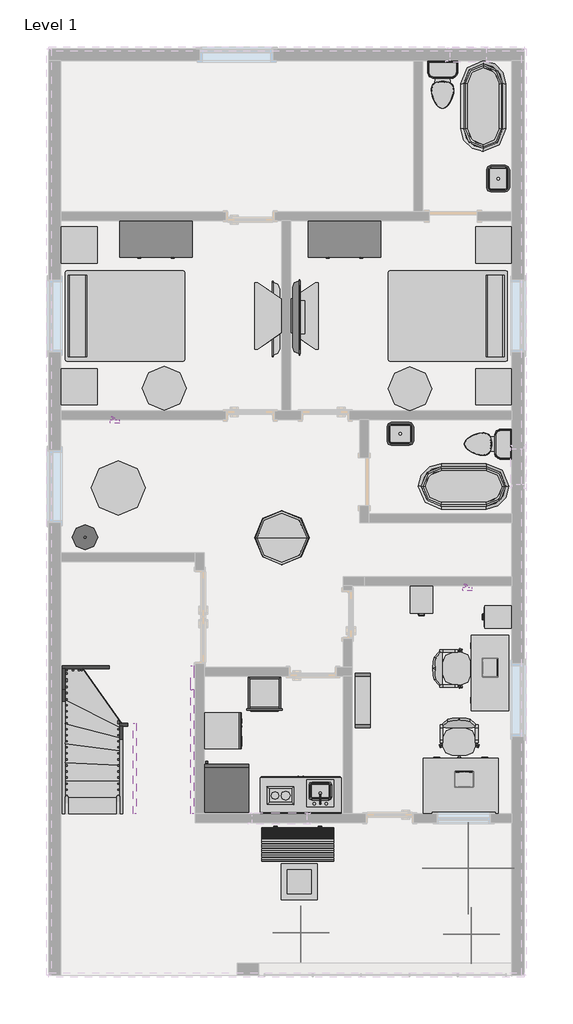
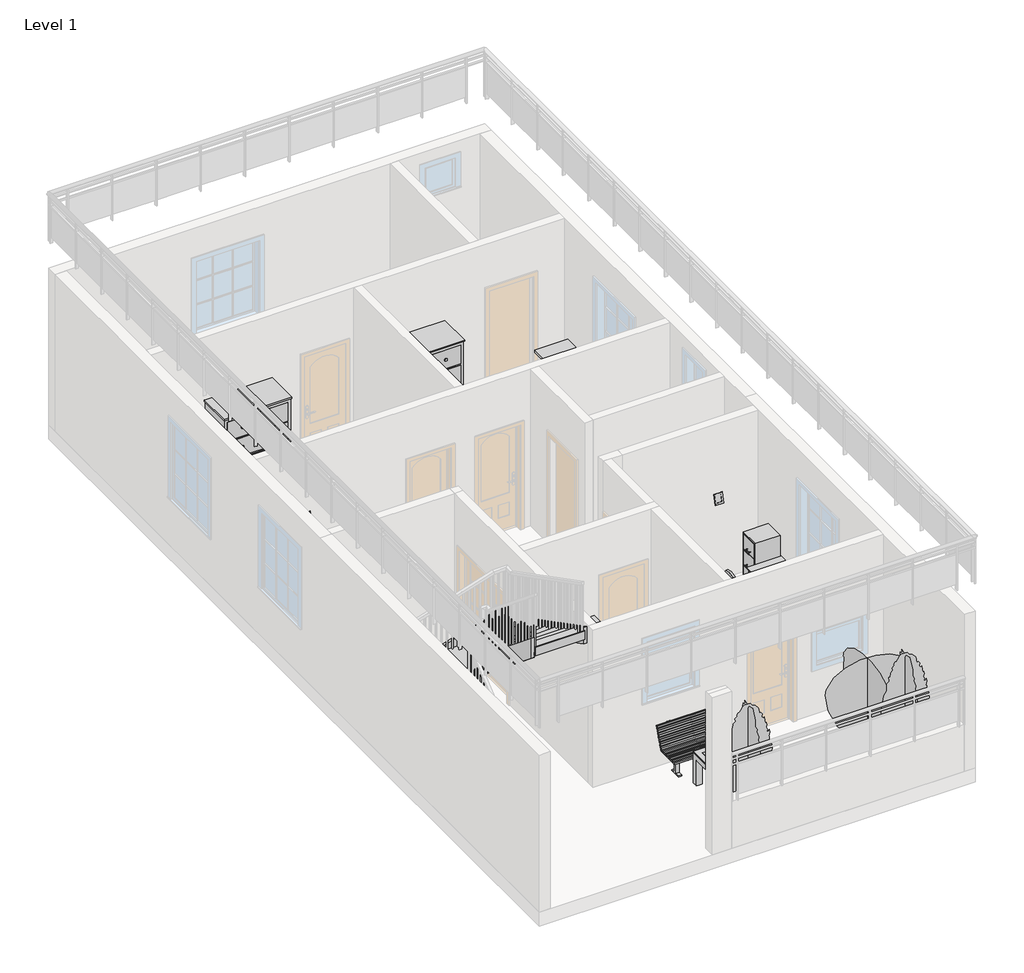
# One storey, part 4 of 4: 25 furniture elements, 9 proxies, 8 flow terminals, 8 members, 4 geographic elements, 1 stair flight.
"""IFC4 building model written with IfcOpenShell, lengths in millimetres."""

from ifc_helpers import new_model, si_unit, frame, origin, place, context, project, spatial, polyline, outline, extrude, transform, mapped, element, save
from components import entourage_4c8cfd20, proxy_fe84b772, proxy_45b28599, proxy_844211aa, proxy_8b8c2dc4, rpc_picture_frame_rpc_picture_frame_c25e3fe9, proxy_a13a33b2, flow_terminal_871c2e40, flow_terminal_d49f872f, flow_terminal_62a433f7, toilet_domestic_3d_toilet_domestic_3d_f7549cf7, toilet_domestic_3d_toilet_domestic_3d_183bbd19, flow_terminal_b374fae2, furniture_e1791683, furniture_552c1472, chair_executive_chair_executive_8d69e98c, furniture_95afb093, furniture_201ebc49, furniture_fdb83c3d, furniture_9fa109b2, furniture_417d203a, furniture_fdf74506, tv_stand_tv_stand_6ce107e5, furniture_b5c51a22, furniture_905aceb5, furniture_b2396e53, furniture_5bc9ed15, furniture_c80d6d9c, geographic_element_d8b57e58, geographic_element_ca6e1e19, rpc_tree_conifer_chinese_juniper_7_1b9786cd, stair_flight_f68c085a

model = new_model("IFC4")

# Units and contexts
model_context = context("Model", 3, world=origin())
ifc_project = project(units=[si_unit("LENGTHUNIT", "METRE", prefix="MILLI")], contexts=[model_context])

# Site, building, storey
site = spatial("IfcSite", under=ifc_project)
building = spatial("IfcBuilding", under=site)
storey = spatial("IfcBuildingStorey", under=building, Name="Level 1", Elevation=0.0)

# Proxies
placement = place(None, origin())
entourage_shape = entourage_4c8cfd20(model_context)
element("IfcBuildingElementProxy", 1, Name="Entourage", at=placement, inside=storey, context=model_context, shape_type="MappedRepresentation", body=[
    mapped(entourage_shape, transform((-6173.1568901, 3253.685263, 736.6), x_axis=(0.0, 1.0, 0.0), y_axis=(-1.0, 0.0, 0.0), z_axis=(0.0, 0.0, 1.0))),
])
element("IfcBuildingElementProxy", 2, Name="Entourage", at=placement, inside=storey, context=model_context, shape_type="MappedRepresentation", body=[
    mapped(entourage_shape, transform((-6573.2068901, 1335.246124, 762.0), x_axis=(-1.0, 0.0, 0.0), y_axis=(0.0, -1.0, 0.0), z_axis=(0.0, 0.0, 1.0))),
])
proxy_shape = proxy_fe84b772(model_context)
element("IfcBuildingElementProxy", 3, Name="Cook Top-2 Unit : 12\" x 18\"", ObjectType="Cook Top-2 Unit : 12\" x 18\"", at=placement, inside=storey, context=model_context, shape_type="MappedRepresentation", body=[
    mapped(proxy_shape, transform((-9695.8816857, 1173.321124, 0.0), x_axis=(0.0, -1.0, 0.0), y_axis=(1.0, 0.0, 0.0), z_axis=(0.0, 0.0, 1.0))),
])
proxy_2_shape = proxy_45b28599(model_context)
element("IfcBuildingElementProxy", 4, Name="Dishwasher : 24\" x 24\" x 34\"", ObjectType="Dishwasher : 24\" x 24\" x 34\"", at=placement, inside=storey, context=model_context, shape_type="MappedRepresentation", body=[
    mapped(proxy_2_shape, transform((-10377.1073253, 1807.0036555, 0.0), x_axis=(0.0, 1.0, 0.0), y_axis=(-1.0, 0.0, 0.0), z_axis=(0.0, 0.0, 1.0))),
])
proxy_3_shape = proxy_844211aa(model_context)
element("IfcBuildingElementProxy", 5, Name="Kitchenette - Small : 54\"", ObjectType="Kitchenette - Small : 54\"", at=placement, inside=storey, context=model_context, shape_type="MappedRepresentation", body=[
    mapped(proxy_3_shape, transform((-9304.0191852, 792.321124, 0.0), x_axis=(-1.0, 0.0, 0.0), y_axis=(0.0, -1.0, 0.0), z_axis=(0.0, 0.0, 1.0))),
])
proxy_4_shape = proxy_8b8c2dc4(model_context)
element("IfcBuildingElementProxy", 6, Name="Oven Double-Built-in : 21 1/2\" x 39 1/4\" x 21\"", ObjectType="Oven Double-Built-in : 21 1/2\" x 39 1/4\" x 21\"", at=placement, inside=storey, context=model_context, shape_type="MappedRepresentation", body=[
    mapped(proxy_4_shape, transform((-9897.1819628, 2683.2552651, 0.0), x_axis=(1.0, 0.0, 0.0), y_axis=(0.0, 1.0, 0.0), z_axis=(0.0, 0.0, 1.0))),
])
rpc_picture_frame_rpc_picture_frame_shape = rpc_picture_frame_rpc_picture_frame_c25e3fe9(model_context)
element("IfcBuildingElementProxy", 7, Name="RPC Picture Frame : RPC Picture Frame", ObjectType="RPC Picture Frame : RPC Picture Frame", at=placement, inside=storey, context=model_context, shape_type="MappedRepresentation", body=[
    mapped(rpc_picture_frame_rpc_picture_frame_shape, transform((-12452.7798632, 7421.721124, 1524.0), x_axis=(1.0, 0.0, 0.0), y_axis=(0.0, 1.0, 0.0), z_axis=(0.0, 0.0, 1.0))),
])
element("IfcBuildingElementProxy", 8, Name="RPC Picture Frame : RPC Picture Frame", ObjectType="RPC Picture Frame : RPC Picture Frame", at=placement, inside=storey, context=model_context, shape_type="MappedRepresentation", body=[
    mapped(rpc_picture_frame_rpc_picture_frame_shape, transform((-6516.8972865, 4602.321124, 1524.0), x_axis=(1.0, 0.0, 0.0), y_axis=(0.0, 1.0, 0.0), z_axis=(0.0, 0.0, 1.0))),
])
proxy_5_shape = proxy_a13a33b2(model_context)
element("IfcBuildingElementProxy", 9, Name="Refrigerator.0001 : 30\" x 32\" RH", ObjectType="Refrigerator.0001 : 30\" x 32\" RH", at=placement, inside=storey, context=model_context, shape_type="MappedRepresentation", body=[
    mapped(proxy_5_shape, transform((-10575.2943901, 1210.2221525, 0.0), x_axis=(-1.0000000000000004, 0.0, 0.0), y_axis=(0.0, -1.0000000000000004, 0.0), z_axis=(0.0, 0.0, 1.0))),
])

# Flow terminals
flow_terminal_shape = flow_terminal_871c2e40(model_context)
element("IfcFlowTerminal", 10, ObjectType="Sink Kitchen-Island : 18\" x 18\"", at=placement, inside=storey, context=model_context, shape_type="MappedRepresentation", body=[
    mapped(flow_terminal_shape, transform((-8976.8676495, 1137.5665251, 0.0), x_axis=(-1.0, 0.0, 0.0), y_axis=(0.0, -1.0, 0.0), z_axis=(0.0, 0.0, 1.0))),
])
flow_terminal_2_shape = flow_terminal_d49f872f(model_context)
element("IfcFlowTerminal", 11, ObjectType="Sink Vanity-Round : 19\" x 19\"", at=placement, inside=storey, context=model_context, shape_type="MappedRepresentation", body=[
    mapped(flow_terminal_2_shape, transform((-12858.3051495, 5532.329344, 609.6), x_axis=(-1.0000000000000004, 0.0, 0.0), y_axis=(0.0, -1.0000000000000004, 0.0), z_axis=(0.0, 0.0, 1.0))),
])
flow_terminal_3_shape = flow_terminal_62a433f7(model_context)
element("IfcFlowTerminal", 12, ObjectType="Sink Vanity-Square : 20\" x 18\"", at=placement, inside=storey, context=model_context, shape_type="MappedRepresentation", body=[
    mapped(flow_terminal_3_shape, transform((-7662.0461307, 7241.5757229, 609.6), x_axis=(1.0, 0.0, 0.0), y_axis=(0.0, 1.0, 0.0), z_axis=(0.0, 0.0, 1.0))),
])
element("IfcFlowTerminal", 13, ObjectType="Sink Vanity-Square : 20\" x 18\"", at=placement, inside=storey, context=model_context, shape_type="MappedRepresentation", body=[
    mapped(flow_terminal_3_shape, transform((-5946.9022912, 11501.4103646, 609.6), x_axis=(0.0, -1.0, 0.0), y_axis=(1.0, 0.0, 0.0), z_axis=(0.0, 0.0, 1.0))),
])
toilet_domestic_3d_toilet_domestic_3d_shape = toilet_domestic_3d_toilet_domestic_3d_f7549cf7(model_context)
toilet_domestic_3d_toilet_domestic_3d_2_shape = toilet_domestic_3d_toilet_domestic_3d_183bbd19(model_context)
element("IfcFlowTerminal", 14, ObjectType="Toilet-Domestic-3D : Toilet-Domestic-3D", at=placement, inside=storey, context=model_context, shape_type="MappedRepresentation", body=[
    mapped(toilet_domestic_3d_toilet_domestic_3d_shape, transform((-6935.1568901, 12972.2250967, 0.0), x_axis=(1.0, 0.0, 0.0), y_axis=(0.0, 1.0, 0.0), z_axis=(0.0, 0.0, 1.0))),
    mapped(toilet_domestic_3d_toilet_domestic_3d_2_shape, transform((-6935.1568901, 12972.2250967, 0.0), x_axis=(1.0, 0.0, 0.0), y_axis=(0.0, 1.0, 0.0), z_axis=(0.0, 0.0, 1.0))),
])
element("IfcFlowTerminal", 15, ObjectType="Toilet-Domestic-3D : Toilet-Domestic-3D", at=placement, inside=storey, context=model_context, shape_type="MappedRepresentation", body=[
    mapped(toilet_domestic_3d_toilet_domestic_3d_shape, transform((-6261.4529174, 7015.321124, 0.0), x_axis=(0.0, -1.0000000000000004, 0.0), y_axis=(1.0000000000000004, 0.0, 0.0), z_axis=(0.0, 0.0, 1.0))),
    mapped(toilet_domestic_3d_toilet_domestic_3d_2_shape, transform((-6261.4529174, 7015.321124, 0.0), x_axis=(0.0, -1.0000000000000004, 0.0), y_axis=(1.0000000000000004, 0.0, 0.0), z_axis=(0.0, 0.0, 1.0))),
])
flow_terminal_4_shape = flow_terminal_b374fae2(model_context)
element("IfcFlowTerminal", 16, ObjectType="Tub-Free Standing-3D : 30\" x 60\"", at=placement, inside=storey, context=model_context, shape_type="MappedRepresentation", body=[
    mapped(flow_terminal_4_shape, transform((-6579.5568901, 6304.121124, 0.0), x_axis=(0.0, -1.0000000000000004, 0.0), y_axis=(1.0000000000000004, 0.0, 0.0), z_axis=(0.0, 0.0, 1.0))),
])
element("IfcFlowTerminal", 17, ObjectType="Tub-Free Standing-3D : 30\" x 60\"", at=placement, inside=storey, context=model_context, shape_type="MappedRepresentation", body=[
    mapped(flow_terminal_4_shape, transform((-6249.3568901, 12704.921124, 0.0), x_axis=(1.0, 0.0, 0.0), y_axis=(0.0, 1.0, 0.0), z_axis=(0.0, 0.0, 1.0))),
])

# Furniture
furniture_shape = furniture_e1791683(model_context)
element("IfcFurniture", 18, ObjectType="Bed-Standard.0001 : Queen 60\" x 79\"", at=placement, inside=storey, context=model_context, shape_type="MappedRepresentation", body=[
    mapped(furniture_shape, transform((-12327.4519721, 8902.8325994, 0.0), x_axis=(0.0, 1.0, 0.0), y_axis=(-1.0, 0.0, 0.0), z_axis=(0.0, 0.0, 1.0))),
])
element("IfcFurniture", 19, ObjectType="Bed-Standard.0001 : Queen 60\" x 79\"", at=placement, inside=storey, context=model_context, shape_type="MappedRepresentation", body=[
    mapped(furniture_shape, transform((-6800.6618081, 9445.8096486, 0.0), x_axis=(0.0, -1.0000000000000002, 0.0), y_axis=(1.0000000000000002, 0.0, 0.0), z_axis=(0.0, 0.0, 1.0))),
])
furniture_2_shape = furniture_552c1472(model_context)
element("IfcFurniture", 20, ObjectType="Cabinet-File 3 Drawer : 15\" x 18\"", at=placement, inside=storey, context=model_context, shape_type="MappedRepresentation", body=[
    mapped(furniture_2_shape, transform((-7162.8604431, 4541.2554242, 0.0), x_axis=(1.0, 0.0, 0.0), y_axis=(0.0, 1.0, 0.0), z_axis=(0.0, 0.0, 1.0))),
])
element("IfcFurniture", 21, ObjectType="Cabinet-File 3 Drawer : 15\" x 18\"", at=placement, inside=storey, context=model_context, shape_type="MappedRepresentation", body=[
    mapped(furniture_2_shape, transform((-5853.22259, 3979.124677, 0.0), x_axis=(0.0, -1.0000000000000004, 0.0), y_axis=(1.0000000000000004, 0.0, 0.0), z_axis=(0.0, 0.0, 1.0))),
])
chair_executive_chair_executive_shape = chair_executive_chair_executive_8d69e98c(model_context)
element("IfcFurniture", 22, ObjectType="Chair-Executive : Chair-Executive", at=placement, inside=storey, context=model_context, shape_type="MappedRepresentation", body=[
    mapped(chair_executive_chair_executive_shape, transform((-6514.7660704, 2055.8670257, 0.0), x_axis=(-1.0000000000000004, 0.0, 0.0), y_axis=(0.0, -1.0000000000000004, 0.0), z_axis=(0.0, 0.0, 1.0))),
])
element("IfcFurniture", 23, ObjectType="Chair-Executive : Chair-Executive", at=placement, inside=storey, context=model_context, shape_type="MappedRepresentation", body=[
    mapped(chair_executive_chair_executive_shape, transform((-6750.9027917, 3379.6234191, 0.0), x_axis=(0.0, -1.0, 0.0), y_axis=(1.0, 0.0, 0.0), z_axis=(0.0, 0.0, 1.0))),
])
furniture_3_shape = furniture_95afb093(model_context)
element("IfcFurniture", 24, ObjectType="Counter Top w Sink Hole : 24\" Depth", at=placement, inside=storey, context=model_context, shape_type="MappedRepresentation", body=[
    mapped(furniture_3_shape, transform((-9837.4191852, 792.321124, 0.0), x_axis=(-1.0, 0.0, 0.0), y_axis=(0.0, -1.0, 0.0), z_axis=(0.0, 0.0, 1.0))),
])
furniture_4_shape = furniture_201ebc49(model_context)
element("IfcFurniture", 25, ObjectType="Credenza : 72\" x 24\"", at=placement, inside=storey, context=model_context, shape_type="MappedRepresentation", body=[
    mapped(furniture_4_shape, transform((-6126.937218, 3221.9768617, 0.0), x_axis=(0.0, -1.0000000000000002, 0.0), y_axis=(1.0000000000000002, 0.0, 0.0), z_axis=(0.0, 0.0, 1.0))),
])
furniture_5_shape = furniture_fdb83c3d(model_context)
element("IfcFurniture", 26, ObjectType="Desk : 72\" x 36\"", at=placement, inside=storey, context=model_context, shape_type="MappedRepresentation", body=[
    mapped(furniture_5_shape, transform((-7239.9568901, 792.321124, 0.0), x_axis=(1.0, 0.0, 0.0), y_axis=(0.0, 1.0, 0.0), z_axis=(0.0, 0.0, 1.0))),
])
furniture_6_shape = furniture_9fa109b2(model_context)
element("IfcFurniture", 27, ObjectType="Dresser : 48\" x 72\" x 24\"", at=placement, inside=storey, context=model_context, shape_type="MappedRepresentation", body=[
    mapped(furniture_6_shape, transform((-8316.9636303, 10832.8840781, 0.0), x_axis=(1.0, 0.0, 0.0), y_axis=(0.0, 1.0, 0.0), z_axis=(0.0, 0.0, 1.0))),
])
element("IfcFurniture", 28, ObjectType="Dresser : 48\" x 72\" x 24\"", at=placement, inside=storey, context=model_context, shape_type="MappedRepresentation", body=[
    mapped(furniture_6_shape, transform((-11491.9636303, 10832.8840781, 0.0), x_axis=(1.0, 0.0, 0.0), y_axis=(0.0, 1.0, 0.0), z_axis=(0.0, 0.0, 1.0))),
])
furniture_7_shape = furniture_417d203a(model_context)
element("IfcFurniture", 29, ObjectType="Shelving : 36\" x 10\" x 72\"", at=placement, inside=storey, context=model_context, shape_type="MappedRepresentation", body=[
    mapped(furniture_7_shape, transform((-8586.1568901, 2697.321124, 0.0), x_axis=(0.0, 0.9999999999999999, 0.0), y_axis=(-0.9999999999999999, 0.0, 0.0), z_axis=(0.0, 0.0, 1.0))),
])
furniture_8_shape = furniture_fdf74506(model_context)
element("IfcFurniture", 30, ObjectType="TV - Flat Screen : 50\"", at=placement, inside=storey, context=model_context, shape_type="MappedRepresentation", body=[
    mapped(furniture_8_shape, transform((-9735.8695203, 9119.5766099, 0.0), x_axis=(0.0, -1.0, 0.0), y_axis=(1.0, 0.0, 0.0), z_axis=(0.0, 0.0, 1.0))),
])
element("IfcFurniture", 31, ObjectType="TV - Flat Screen : 50\"", at=placement, inside=storey, context=model_context, shape_type="MappedRepresentation", body=[
    mapped(furniture_8_shape, transform((-9403.2339556, 9152.8656382, 609.6), x_axis=(0.0, 1.0, 0.0), y_axis=(-1.0, 0.0, 0.0), z_axis=(0.0, 0.0, 1.0))),
])
tv_stand_tv_stand_shape = tv_stand_tv_stand_6ce107e5(model_context)
element("IfcFurniture", 32, ObjectType="TV Stand : TV Stand", at=placement, inside=storey, context=model_context, shape_type="MappedRepresentation", body=[
    mapped(tv_stand_tv_stand_shape, transform((-9640.2568901, 9299.5091261, 609.6), x_axis=(0.0, -1.0000000000000004, 0.0), y_axis=(1.0000000000000004, 0.0, 0.0), z_axis=(0.0, 0.0, 1.0))),
])
element("IfcFurniture", 33, ObjectType="TV Stand : TV Stand", at=placement, inside=storey, context=model_context, shape_type="MappedRepresentation", body=[
    mapped(tv_stand_tv_stand_shape, transform((-9487.8568901, 9049.133122, 0.0), x_axis=(0.0, 1.0000000000000002, 0.0), y_axis=(-1.0000000000000002, 0.0, 0.0), z_axis=(0.0, 0.0, 1.0))),
])
furniture_9_shape = furniture_b5c51a22(model_context)
element("IfcFurniture", 34, ObjectType="Table-Coffee : 24\" x 24\" x 24\"", at=placement, inside=storey, context=model_context, shape_type="MappedRepresentation", body=[
    mapped(furniture_9_shape, transform((-9366.4226568, -445.8899538, 0.0), x_axis=(1.0, 0.0, 0.0), y_axis=(0.0, 1.0, 0.0), z_axis=(0.0, 0.0, 1.0))),
])
furniture_10_shape = furniture_905aceb5(model_context)
element("IfcFurniture", 35, ObjectType="Table-Dining Round w Chairs : 36\" Diameter", at=placement, inside=storey, context=model_context, shape_type="MappedRepresentation", body=[
    mapped(furniture_10_shape, transform((-12499.8388573, 6463.5998126, 0.0), x_axis=(1.0, 0.0, 0.0), y_axis=(0.0, 1.0, 0.0), z_axis=(0.0, 0.0, 1.0))),
])
furniture_11_shape = furniture_b2396e53(model_context)
element("IfcFurniture", 36, ObjectType="Table-Ellipse : 72\" x 36\"", at=placement, inside=storey, context=model_context, shape_type="MappedRepresentation", body=[
    mapped(furniture_11_shape, transform((-11621.4568901, 7955.121124, 0.0), x_axis=(-1.0000000000000004, 0.0, 0.0), y_axis=(0.0, -1.0000000000000004, 0.0), z_axis=(0.0, 0.0, 1.0))),
])
element("IfcFurniture", 37, ObjectType="Table-Ellipse : 72\" x 36\"", at=placement, inside=storey, context=model_context, shape_type="MappedRepresentation", body=[
    mapped(furniture_11_shape, transform((-7483.7789881, 7947.2120203, 0.0), x_axis=(1.0000000000000009, 0.0, 0.0), y_axis=(0.0, 1.0000000000000009, 0.0), z_axis=(0.0, 0.0, 1.0))),
])
furniture_12_shape = furniture_5bc9ed15(model_context)
element("IfcFurniture", 38, ObjectType="Table-Night Stand : 24\" x 24\" x 30\"", at=placement, inside=storey, context=model_context, shape_type="MappedRepresentation", body=[
    mapped(furniture_12_shape, transform((-13365.0905204, 7675.721124, 0.0), x_axis=(1.0, 0.0, 0.0), y_axis=(0.0, 1.0, 0.0), z_axis=(0.0, 0.0, 1.0))),
])
element("IfcFurniture", 39, ObjectType="Table-Night Stand : 24\" x 24\" x 30\"", at=placement, inside=storey, context=model_context, shape_type="MappedRepresentation", body=[
    mapped(furniture_12_shape, transform((-13365.0905204, 10063.321124, 0.0), x_axis=(1.0, 0.0, 0.0), y_axis=(0.0, 1.0, 0.0), z_axis=(0.0, 0.0, 1.0))),
])
element("IfcFurniture", 40, ObjectType="Table-Night Stand : 24\" x 24\" x 30\"", at=placement, inside=storey, context=model_context, shape_type="MappedRepresentation", body=[
    mapped(furniture_12_shape, transform((-6380.0905204, 10063.321124, 0.0), x_axis=(1.0, 0.0, 0.0), y_axis=(0.0, 1.0, 0.0), z_axis=(0.0, 0.0, 1.0))),
])
element("IfcFurniture", 41, ObjectType="Table-Night Stand : 24\" x 24\" x 30\"", at=placement, inside=storey, context=model_context, shape_type="MappedRepresentation", body=[
    mapped(furniture_12_shape, transform((-6380.0905204, 7675.721124, 0.0), x_axis=(1.0, 0.0, 0.0), y_axis=(0.0, 1.0, 0.0), z_axis=(0.0, 0.0, 1.0))),
])
furniture_13_shape = furniture_c80d6d9c(model_context)
element("IfcFurniture", 42, ObjectType="Table-Round : 36\" Diameter", at=placement, inside=storey, context=model_context, shape_type="MappedRepresentation", body=[
    mapped(furniture_13_shape, transform((-9640.2568901, 5440.521124, 0.0), x_axis=(1.0, 0.0, 0.0), y_axis=(0.0, 1.0, 0.0), z_axis=(0.0, 0.0, 1.0))),
])

# Geographic elements
geographic_element_shape = geographic_element_d8b57e58(model_context)
element("IfcGeographicElement", 43, ObjectType="Park Bench : 72\"", at=placement, inside=storey, context=model_context, shape_type="MappedRepresentation", body=[
    mapped(geographic_element_shape, transform((-9373.5568901, 309.721124, 0.0), x_axis=(1.0, 0.0, 0.0), y_axis=(0.0, 1.0, 0.0), z_axis=(0.0, 0.0, 1.0))),
])
geographic_element_2_shape = geographic_element_ca6e1e19(model_context)
element("IfcGeographicElement", 44, ObjectType="RPC Shrub : Burning Bush 4'-6\"", at=placement, inside=storey, context=model_context, shape_type="MappedRepresentation", body=[
    mapped(geographic_element_2_shape, transform((-6503.3568901, -122.078876, 0.0), x_axis=(1.0, 0.0, 0.0), y_axis=(0.0, 1.0, 0.0), z_axis=(0.0, 0.0, 1.0))),
])
rpc_tree_conifer_chinese_juniper_7_shape = rpc_tree_conifer_chinese_juniper_7_1b9786cd(model_context)
element("IfcGeographicElement", 45, ObjectType="RPC Tree - Conifer : Chinese Juniper - 7'", at=placement, inside=storey, context=model_context, shape_type="MappedRepresentation", body=[
    mapped(rpc_tree_conifer_chinese_juniper_7_shape, transform((-6452.7535612, -1239.678876, 0.0), x_axis=(1.0, 0.0, 0.0), y_axis=(0.0, 1.0, 0.0), z_axis=(0.0, 0.0, 1.0))),
])
element("IfcGeographicElement", 46, ObjectType="RPC Tree - Conifer : Chinese Juniper - 7'", at=placement, inside=storey, context=model_context, shape_type="MappedRepresentation", body=[
    mapped(rpc_tree_conifer_chinese_juniper_7_shape, transform((-9322.9535612, -1214.278876, 0.0), x_axis=(1.0, 0.0, 0.0), y_axis=(0.0, 1.0, 0.0), z_axis=(0.0, 0.0, 1.0))),
])

# Members
element("IfcMember", 47, ObjectType="Stringer - 2\" Width", at=placement, inside=storey, context=model_context, shape_type="SweptSolid", body=[
    extrude(outline(polyline([(792.321124, 0.0), (792.321124, 229.639954), (2879.7383157, 1305.3956453), (2879.7383157, 962.500629), (1012.0834416, 0.0), (792.321124, 0.0)])), frame((-13335.9568901, 0.0, 0.0), z_axis=(1.0, 0.0, 0.0), x_axis=(0.0, 1.0, 0.0)), (0.0, 0.0, 1.0), 50.8),
])
element("IfcMember", 48, ObjectType="Stringer - 2\" Width", at=placement, inside=storey, context=model_context, shape_type="SweptSolid", body=[
    extrude(outline(polyline([(-13285.1568901, 2879.7383157), (-13335.9568901, 2879.7383157), (-13335.9568901, 3234.4528159), (-13285.1568901, 3234.4528159), (-13285.1568901, 2879.7383157)])), frame((0.0, 0.0, 962.500629), z_axis=(0.0, 0.0, 1.0), x_axis=(1.0, 0.0, 0.0)), (0.0, 0.0, 1.0), 342.8950162),
])
element("IfcMember", 49, ObjectType="Stringer - 2\" Width", at=placement, inside=storey, context=model_context, shape_type="SweptSolid", body=[
    extrude(outline(polyline([(1289.0952212, -13335.9568901), (1000.5956453, -13335.9568901), (1000.5956453, -13166.4344071), (1638.9682298, -11176.9568901), (1969.9972697, -11176.9568901), (1969.9972697, -11213.9370074), (1289.0952212, -13335.9568901)])), frame((0.0, 3234.4528159, 0.0), z_axis=(0.0, 1.0, 0.0), x_axis=(0.0, 0.0, 1.0)), (0.0, 0.0, 1.0), 50.8),
])
element("IfcMember", 50, ObjectType="Stringer - 2\" Width", at=placement, inside=storey, context=model_context, shape_type="SweptSolid", body=[
    extrude(outline(polyline([(-11176.9568901, 3285.2528159), (-11126.1568901, 3285.2528159), (-11126.1568901, 2879.7383157), (-11176.9568901, 2879.7383157), (-11176.9568901, 3285.2528159)])), frame((0.0, 0.0, 1649.8904473), z_axis=(0.0, 0.0, 1.0), x_axis=(1.0, 0.0, 0.0)), (0.0, 0.0, 1.0), 320.1068224),
])
element("IfcMember", 51, ObjectType="Stringer - 2\" Width", at=placement, inside=storey, context=model_context, shape_type="SweptSolid", body=[
    extrude(outline(polyline([(2879.7383157, 1969.9972697), (2879.7383157, 1649.8904473), (792.321124, 2725.6461385), (792.321124, 3045.7529609), (2879.7383157, 1969.9972697)])), frame((-11176.9568901, 0.0, 0.0), z_axis=(1.0, 0.0, 0.0), x_axis=(0.0, 1.0, 0.0)), (0.0, 0.0, 1.0), 50.8),
])
element("IfcMember", 52, ObjectType="Stringer - 2\" Width", at=placement, inside=storey, context=model_context, shape_type="SweptSolid", body=[
    extrude(outline(polyline([(792.321124, 0.0), (792.321124, 176.1764461), (2269.2528159, 1380.418648), (2269.2528159, 987.1410923), (1058.5827686, 0.0), (792.321124, 0.0)])), frame((-12370.7568901, 0.0, 0.0), z_axis=(1.0, 0.0, 0.0), x_axis=(0.0, 1.0, 0.0)), (0.0, 0.0, 1.0), 50.8),
])
element("IfcMember", 53, ObjectType="Stringer - 2\" Width", at=placement, inside=storey, context=model_context, shape_type="SweptSolid", body=[
    extrude(outline(polyline([(1573.2682978, -12370.7568901), (1028.5617647, -12370.7568901), (1028.5617647, -12336.5146728), (1360.465107, -12142.1568901), (1926.1409689, -12142.1568901), (1926.1409689, -12164.1197727), (1573.2682978, -12370.7568901)])), frame((0.0, 2269.2528159, 0.0), z_axis=(0.0, 1.0, 0.0), x_axis=(0.0, 0.0, 1.0)), (0.0, 0.0, 1.0), 50.8),
])
element("IfcMember", 54, ObjectType="Stringer - 2\" Width", at=placement, inside=storey, context=model_context, shape_type="SweptSolid", body=[
    extrude(outline(polyline([(2320.0528159, 1926.1409689), (2320.0528159, 1532.8634131), (792.321124, 2778.5262875), (792.321124, 3171.8038432), (2320.0528159, 1926.1409689)])), frame((-12142.1568901, 0.0, 0.0), z_axis=(1.0, 0.0, 0.0), x_axis=(0.0, 1.0, 0.0)), (0.0, 0.0, 1.0), 50.8),
])

# Stair flight
stair_flight_shape = stair_flight_f68c085a(model_context)
element("IfcStairFlight", 55, ObjectType="2\" Tread 1\" Nosing 1/4\" Riser", at=placement, inside=storey, context=model_context, shape_type="MappedRepresentation", body=[
    mapped(stair_flight_shape, transform((0.0, 0.0, 0.0), x_axis=(1.0, 0.0, 0.0), y_axis=(0.0, 1.0, 0.0), z_axis=(0.0, 0.0, 1.0))),
])

save(model, "model.ifc")

# Revit data of these elements
# Type
#   built-in parameter 1005195 = "RPC-16-N04H-AQSP-D1N4-43SU-6GKQ-C3KU-1C"
#   Height = 0
# Type "Cook Top-2 Unit : 12\" x 18\""
#   Assembly Code = "E1090400"
#   Counter Height = 3' - 0"
#   Depth = 1' - 6"
#   Width = 1' - 0"
#   Burner Material = Steel, Chrome Plated
#   Cooktop Material = Steel, Polished
#   Default Elevation = 0
# Type "Dishwasher : 24\" x 24\" x 34\""
#   Label = "DW"
#   Assembly Code = "E1090400"
#   Depth = 2' - 0"
#   Height = 2' - 10"
#   Width = 2' - 0"
#   Dishwasher Material = Steel, Paint Finish, Ivory, Glossy
#   Panel Face Material = Plastic, Opaque Black
#   Default Elevation = 0
# Type "Kitchenette - Small : 54\""
#   Assembly Code = "E1090400"
#   Width = 4' - 6"
#   Height = 2' - 10 1/2"
#   Depth = 2' - 0"
#   Toe Depth = 0' - 3"
#   Toe Height = 0' - 3 1/2"
#   Cabinet Material = Cabinets
#   Door/Drawer Material = Cabinets
#   Handle Material = Cabinets - Handles
#   Default Elevation = 0
# Type "Oven Double-Built-in : 21 1/2\" x 39 1/4\" x 21\""
#   Label = "OVEN"
#   Assembly Code = "E1090400"
#   Depth = 1' - 9"
#   Height = 3' - 3 1/4"
#   Width = 1' - 9 1/2"
#   Oven Material = Metal - Stainless Steel, Polished
#   Default Elevation = 0
# Type "RPC Picture Frame : RPC Picture Frame"
#   built-in parameter 1005198 = "{2, 15},{39, RPC-16-8M5E-0H3T-F0AH-3U0K-JLQ7-G28B-AU},{1, 0},{1, 0},{2, 19},{1, 8},{5, Color},{1, 0},{1, 0},{3, 0.8},{3, 0.8},{3, 0.8},{1, 8},{7, BBoxMin},{1, 0},{1, 0},{1, 0},{1, 0},{1, 0},{1, 8},{7, BBoxMax},{1, 0},{1, 0},{1, 0},{1, 0},{1, 0},{2, 11},{9, RPCTypeId},{1, 0},{1, 0},{39, RPC-16-8M5E-0H3T-F0AH-3U0K-JLQ7-G28B-AU},{1, 6},{14, RPCPlantHeight},{1, 0},{1, 0},{5, 0.625},{2, 11},{7, keyword},{1, 0},{1, 0},{33, :RPCs:Office Clutter:Geometry:RPC},{2, 11},{8, category},{1, 0},{1, 0},{14, Office Clutter},{2, 11},{12, LocalizedUID},{1, 0},{1, 0},{13, Picture Frame},{2, 14},{6, Height},{1, 0},{1, 0},{5, 0.625},{1, 2},{16, Cast Reflections},{1, 0},{1, 0},{1, 0},{1, 2},{8, Portrait},{1, 0},{1, 0},{1, 1},{1, 2},{5, Stand},{1, 0},{1, 0},{1, 1},{2, 11},{10, RPCL_Frame},{1, 0},{1, 0},{5, Frame},{1, 4},{14, Frame Material},{1, 0},{1, 0},{1, 0},{2, 11},{12, RPCL_Picture},{1, 0},{1, 0},{7, Picture},{2, 11},{15, Picture Preview},{1, 0},{1, 0},{65, __RPC:/object data/textures/object/Photo/Photo0/textures/Portrait},{2, 11},{17, i_Picture Preview},{1, 0},{1, 0},{0, },{1, 2},{18, Use Custom Picture},{1, 0},{1, 0},{1, 0},{2, 11},{17, Picture File Name},{1, 0},{1, 0},{0, },{21, assetlibrary_base.fbx},{1, 5},"
#   built-in parameter 1005195 = "RPC-16-8M5E-0H3T-F0AH-3U0K-JLQ7-G28B-AU"
#   Height = 0
# Type "Refrigerator.0001 : 30\" x 32\" RH"
#   Label = "REF."
#   Assembly Code = "E1090400"
#   Depth = 2' - 7 3/4"
#   Handle = 2' - 3"
#   Height = 5' - 10"
#   Rear Clearance = 0' - 2"
#   Top Door Height = 1' - 8"
#   Width = 2' - 5 3/8"
#   Material = Steel, Paint Finish, Ivory, Glossy
#   Default Elevation = 0
# Type "Sink Kitchen-Island : 18\" x 18\""
#   Assembly Code = "D2010410"
#   Counter Height = 3' - 0"
#   Depth = 1' - 6"
#   Width = 1' - 6"
#   Faucet Material = Steel, Polished
#   Sink Material = Steel, Polished
#   Default Elevation = 0
# Type "Sink Vanity-Round : 19\" x 19\""
#   Assembly Code = "D2010400"
#   Top Of Counter = 2' - 7"
#   Basin Material = Porcelain, Linen
#   Faucet Material = Steel, Polished
#   Default Elevation = 0
# Type "Sink Vanity-Square : 20\" x 18\""
#   Assembly Code = "D2010400"
#   Counter Height = 2' - 7"
#   Depth = 1' - 6"
#   Width = 1' - 8"
#   Basin Material = Porcelain, Linen
#   Faucet Material = Steel, Polished
#   Default Elevation = 0
# Type "Toilet-Domestic-3D : Toilet-Domestic-3D"
#   Assembly Code = "D2010110"
#   Toilet - Bowl/Basin Material = Porcelain, Linen
#   Toilet - Seat Material = Laminate, Linen, Matte
#   Default Elevation = 0
# Type "Tub-Free Standing-3D : 30\" x 60\""
#   Assembly Code = "D2010110"
#   Height = 1' - 6"
#   Length = 5' - 0"
#   Width = 2' - 6"
#   Tub Material = Porcelain, Ivory
#   Default Elevation = 0
# Type "Bed-Standard.0001 : Queen 60\" x 79\""
#   Assembly Code = "E2020200"
#   Length = 6' - 7"
#   Width = 5' - 0"
#   Leg Material = Steel, Chrome Plated
#   Mattress Material = Linen, White
#   Default Elevation = 0
# Type "Cabinet-File 3 Drawer : 15\" x 18\""
#   Assembly Code = "E2020200"
#   Depth = 1' - 6"
#   Height = 3' - 5"
#   Width = 1' - 3"
#   Cabinet Material = Steel, Paint Finish, Ivory, Glossy
#   Handle Material = Steel, Chrome Plated
#   Default Elevation = 0
# Type "Chair-Executive : Chair-Executive"
#   Assembly Code = "E2020200"
#   Base/Arms Material = Plastic, Opaque Black
#   Casters Material = Plastic, Opaque Black
#   Seat/Back Material = Textile - Slate Blue
#   Default Elevation = 0
# Type "Counter Top w Sink Hole : 24\" Depth"
#   Assembly Code = "C1030400"
#   Counter Thickness = 0' - 1 1/2"
#   Depth [instance default] = 2' - 1"
#   Height = 3' - 0"
#   Length [instance default] = 8' - 0"
#   Sink Location [instance default] = 2' - 0"
#   Sink Location To Wall [instance default] = 0' - 6"
#   Sink Opening Depth [instance default] = 1' - 3"
#   Sink Opening Width [instance default] = 2' - 3"
#   Counter Top Material = none
#   Default Elevation = 0
# Type "Credenza : 72\" x 24\""
#   Assembly Code = "E2020200"
#   Depth = 2' - 0"
#   Height = 2' - 5"
#   Width = 4' - 0"
#   Body Material = Laminate, Ivory, Matte
#   Handles/Legs Material = Steel, Chrome Plated
#   Top Material = Cherry
#   Default Elevation = 0
# Type "Desk : 72\" x 36\""
#   Assembly Code = "E2020200"
#   Depth = 3' - 0"
#   Height = 2' - 6"
#   Leg Height = 0' - 6"
#   Width = 4' - 0"
#   Body Material = Laminate, Ivory, Matte
#   Handle/Leg Material = Steel, Chrome Plated
#   Top Material = Cherry
#   Default Elevation = 0
# Type "Dresser : 48\" x 72\" x 24\""
#   Assembly Code = "E2020200"
#   Depth = 2' - 0"
#   Height = 6' - 0"
#   Width = 4' - 0"
#   Dresser Material = Laminate - Ivory, Glossy
#   Drawer Material = Laminate, Ivory, Matte
#   Knob Material = Cherry
#   Default Elevation = 0
# Type "Shelving : 36\" x 10\" x 72\""
#   Assembly Code = "E2020200"
#   Depth = 0' - 10"
#   Height = 6' - 0"
#   Width = 3' - 0"
#   Shelving Unit Material = Birch
#   Default Elevation = 0
# Type "TV - Flat Screen : 50\""
#   SinAng = 0' - 0.0193"
#   L = 3' - 7.57782"
#   H = 2' - 0.51477"
#   Thickness = 0' - 4.33071"
#   Diagonal = 4' - 2"
#   CosAng = 0' - 0.03431"
#   Stand [instance default] = yes
#   Default Elevation = 0
# Type "TV Stand : TV Stand"
#   Depth = 1' - 6"
#   Width = 3' - 8"
#   Height = 1' - 7 1/2"
#   Finish = Melamine - Gray
#   Default Elevation = 0
# Type "Table-Coffee : 24\" x 24\" x 24\""
#   Assembly Code = "E2020200"
#   Height = 2' - 0"
#   Length = 2' - 0"
#   Width = 2' - 0"
#   Top Material = none
#   Frame Material = none
#   Default Elevation = 0
# Type "Table-Dining Round w Chairs : 36\" Diameter"
#   Assembly Code = "E2020200"
#   Radius = 1' - 6"
#   Diameter = 3' - 0"
#   Height = 2' - 6"
#   Chairs = 4
#   Base Material = Pine
#   Top Material = Laminate, Linen, Matte
#   Default Elevation = 0
# Type "Table-Ellipse : 72\" x 36\""
#   Assembly Code = "E2020200"
#   Half Width = 1' - 2 1/2"
#   Half Length = 1' - 2 1/2"
#   Height = 2' - 6"
#   Length = 2' - 5"
#   Width = 2' - 5"
#   Base Material = Birch
#   Top Material = Laminate - Black
#   Default Elevation = 0
# Type "Table-Night Stand : 24\" x 24\" x 30\""
#   Assembly Code = "E2020200"
#   Depth = 2' - 0"
#   Height = 2' - 6"
#   Width = 2' - 0"
#   Base Material = Birch
#   Top Material = Laminate, Ivory, Matte
#   Default Elevation = 0
# Type "Table-Round : 36\" Diameter"
#   Assembly Code = "E2020200"
#   Base Radius = 0' - 10"
#   Height = 2' - 6"
#   Radius = 1' - 6"
#   Base Material = Steel, Chrome Plated
#   Top Material = Birch
#   Default Elevation = 0
# Type "Park Bench : 72\""
#   Length = 4' - 0"
#   Seat Material = Wood - Teak
#   Frame Material = Steel, Paint Finish, Dark Gray, Matte
# Type "RPC Shrub : Burning Bush 4'-6\""
#   Type Comments = "Burning Bush"
#   built-in parameter 1005198 = "{2, 15},{39, RPC-16-FVGW-0UXX-7JA7-N000-ST1L-LVER-AU},{1, 0},{1, 0},{2, 13},{1, 8},{5, Color},{1, 0},{1, 0},{3, 0.8},{3, 0.8},{3, 0.8},{1, 8},{7, BBoxMin},{1, 0},{1, 0},{1, 0},{1, 0},{1, 0},{1, 8},{7, BBoxMax},{1, 0},{1, 0},{1, 0},{1, 0},{1, 0},{2, 11},{9, RPCTypeId},{1, 0},{1, 0},{39, RPC-16-FVGW-0UXX-7JA7-N000-ST1L-LVER-AU},{1, 6},{14, RPCPlantHeight},{1, 0},{1, 0},{3, 4.5},{2, 11},{7, keyword},{1, 0},{1, 0},{35, :RPCs:Shrubs & Grasses:Geometry:RPC},{2, 11},{8, category},{1, 0},{1, 0},{16, Shrubs & Grasses},{2, 11},{12, LocalizedUID},{1, 0},{1, 0},{12, Burning Bush},{2, 14},{6, Height},{1, 0},{1, 0},{3, 4.5},{1, 2},{16, Cast Reflections},{1, 0},{1, 0},{1, 0},{1, 2},{12, Cast Shadows},{1, 0},{1, 0},{1, 1},{1, 2},{9, Lock View},{1, 0},{1, 0},{1, 0},{1, 4},{5, ViewC},{1, 0},{1, 0},{1, 0},{21, assetlibrary_base.fbx},{1, 5},"
#   built-in parameter 1005195 = "RPC-16-FVGW-0UXX-7JA7-N000-ST1L-LVER-AU"
#   Assembly Code = "G2050500"
#   Height = 4' - 6"
#   Default Elevation = 0
# Type "RPC Tree - Conifer : Chinese Juniper - 7'"
#   built-in parameter 1005198 = "{2, 15},{39, RPC-16-FUM3-UUQ0-UBF0-N000-ST1L-LVER-AU},{1, 0},{1, 0},{2, 13},{1, 8},{5, Color},{1, 0},{1, 0},{3, 0.8},{3, 0.8},{3, 0.8},{1, 8},{7, BBoxMin},{1, 0},{1, 0},{1, 0},{1, 0},{1, 0},{1, 8},{7, BBoxMax},{1, 0},{1, 0},{1, 0},{1, 0},{1, 0},{2, 11},{9, RPCTypeId},{1, 0},{1, 0},{39, RPC-16-FUM3-UUQ0-UBF0-N000-ST1L-LVER-AU},{1, 6},{14, RPCPlantHeight},{1, 0},{1, 0},{1, 7},{2, 11},{7, keyword},{1, 0},{1, 0},{34, :RPCs:Trees [General]:Geometry:RPC},{2, 11},{8, category},{1, 0},{1, 0},{15, Trees [General]},{2, 11},{12, LocalizedUID},{1, 0},{1, 0},{15, Chinese Juniper},{2, 14},{6, Height},{1, 0},{1, 0},{1, 7},{1, 2},{16, Cast Reflections},{1, 0},{1, 0},{1, 0},{1, 2},{12, Cast Shadows},{1, 0},{1, 0},{1, 1},{1, 2},{9, Lock View},{1, 0},{1, 0},{1, 0},{1, 4},{5, ViewC},{1, 0},{1, 0},{1, 0},{21, assetlibrary_base.fbx},{1, 5},"
#   built-in parameter 1005195 = "RPC-16-FUM3-UUQ0-UBF0-N000-ST1L-LVER-AU"
#   Type Comments = "Chinese Juniper"
#   Assembly Code = "G2050500"
#   Height = 7' - 0"
#   Description = (empty or 0)
#   Default Elevation = 0
# Elements 1, 2 (IfcBuildingElementProxy)
#   Phase Created = New Construction
# Element 3 (IfcBuildingElementProxy, "Cook Top-2 Unit : 12\" x 18\"")
#   Phase Created = New Construction
#   Materials on its faces: "Steel, Chrome Plated", "Steel, Polished"
# Element 4 (IfcBuildingElementProxy, "Dishwasher : 24\" x 24\" x 34\"")
#   Phase Created = New Construction
#   Materials on its faces: "Steel, Paint Finish, Ivory, Glossy", "Plastic, Opaque Black"
# Element 5 (IfcBuildingElementProxy, "Kitchenette - Small : 54\"")
#   Phase Created = New Construction
#   Materials on its faces: "Cabinets", "Cabinets - Handles"
# Element 6 (IfcBuildingElementProxy, "Oven Double-Built-in : 21 1/2\" x 39 1/4\" x 21\"")
#   Phase Created = New Construction
#   Materials on its faces: "Steel", "Metal - Stainless Steel, Polished", "Glass"
# Elements 7, 8 (IfcBuildingElementProxy, "RPC Picture Frame : RPC Picture Frame")
#   Phase Created = New Construction
# Element 9 (IfcBuildingElementProxy, "Refrigerator.0001 : 30\" x 32\" RH")
#   Phase Created = New Construction
#   Materials on its faces: "Steel, Paint Finish, Ivory, Glossy", "Steel, Chrome Plated"
# Element 10 (IfcFlowTerminal, "Sink Kitchen-Island : 18\" x 18\"")
#   Mark = "7"
#   Phase Created = New Construction
#   Materials on its faces: "Steel, Polished"
# Element 11 (IfcFlowTerminal, "Sink Vanity-Round : 19\" x 19\"")
#   Mark = "8"
#   Phase Created = New Construction
#   Materials on its faces: "Porcelain, Linen", "Steel, Polished"
# Element 12 (IfcFlowTerminal, "Sink Vanity-Square : 20\" x 18\"")
#   Mark = "5"
#   Phase Created = New Construction
#   Materials on its faces: "Porcelain, Linen", "Steel, Polished"
# Element 13 (IfcFlowTerminal, "Sink Vanity-Square : 20\" x 18\"")
#   Mark = "6"
#   Phase Created = New Construction
#   Materials on its faces: "Porcelain, Linen", "Steel, Polished"
# Element 14 (IfcFlowTerminal, "Toilet-Domestic-3D : Toilet-Domestic-3D")
#   Mark = "1"
#   Phase Created = New Construction
#   Materials on its faces: "Porcelain, Linen", "Laminate, Linen, Matte"
# Element 15 (IfcFlowTerminal, "Toilet-Domestic-3D : Toilet-Domestic-3D")
#   Mark = "2"
#   Phase Created = New Construction
#   Materials on its faces: "Porcelain, Linen", "Laminate, Linen, Matte"
# Element 16 (IfcFlowTerminal, "Tub-Free Standing-3D : 30\" x 60\"")
#   Mark = "3"
#   Phase Created = New Construction
#   Materials on its faces: "Porcelain, Ivory"
# Element 17 (IfcFlowTerminal, "Tub-Free Standing-3D : 30\" x 60\"")
#   Mark = "4"
#   Phase Created = New Construction
#   Materials on its faces: "Porcelain, Ivory"
# Elements 18, 19 (IfcFurniture, "Bed-Standard.0001 : Queen 60\" x 79\"")
#   Phase Created = New Construction
#   Materials on its faces: "Linen, White", "Steel, Chrome Plated"
# Elements 20, 21 (IfcFurniture, "Cabinet-File 3 Drawer : 15\" x 18\"")
#   Phase Created = New Construction
#   Materials on its faces: "Steel, Chrome Plated", "Steel, Paint Finish, Ivory, Glossy"
# Elements 22, 23 (IfcFurniture, "Chair-Executive : Chair-Executive")
#   Phase Created = New Construction
#   Materials on its faces: "Plastic, Opaque Black", "Textile - Slate Blue"
# Element 24 (IfcFurniture, "Counter Top w Sink Hole : 24\" Depth")
#   Sink Opening Depth = 1' - 3"
#   Sink Location To Wall = 0' - 6"
#   Length = 4' - 6"
#   Sink Location = 1' - 2"
#   Sink Opening Width = 1' - 4"
#   Depth = 2' - 0"
#   Phase Created = New Construction
#   Materials on its faces: "Counter Top"
# Element 25 (IfcFurniture, "Credenza : 72\" x 24\"")
#   Phase Created = New Construction
#   Materials on its faces: "Steel, Chrome Plated", "Laminate, Ivory, Matte", "Cherry"
# Element 26 (IfcFurniture, "Desk : 72\" x 36\"")
#   Phase Created = New Construction
#   Materials on its faces: "Steel, Chrome Plated", "Laminate, Ivory, Matte", "Cherry"
# Elements 27, 28 (IfcFurniture, "Dresser : 48\" x 72\" x 24\"")
#   Phase Created = New Construction
#   Materials on its faces: "Laminate, Ivory, Matte", "Cherry", "Laminate - Ivory, Glossy"
# Element 29 (IfcFurniture, "Shelving : 36\" x 10\" x 72\"")
#   Phase Created = New Construction
#   Materials on its faces: "Birch"
# Elements 30, 31 (IfcFurniture, "TV - Flat Screen : 50\"")
#   Stand = yes
#   Phase Created = New Construction
#   Materials on its faces: "TV - Black", "TV - Glass", "TV - Screen"
# Elements 32, 33 (IfcFurniture, "TV Stand : TV Stand")
#   Phase Created = New Construction
#   Materials on its faces: "Melamine - Gray", "Glass - Shelves"
# Element 34 (IfcFurniture, "Table-Coffee : 24\" x 24\" x 24\"")
#   Phase Created = New Construction
#   Materials on its faces: "Glass - Clear, Grey"
# Element 35 (IfcFurniture, "Table-Dining Round w Chairs : 36\" Diameter")
#   Phase Created = New Construction
#   Materials on its faces: "Pine", "Laminate, Linen, Matte"
# Elements 36, 37 (IfcFurniture, "Table-Ellipse : 72\" x 36\"")
#   Phase Created = New Construction
#   Materials on its faces: "Birch", "Laminate - Black"
# Elements 38, 39, 40, 41 (IfcFurniture, "Table-Night Stand : 24\" x 24\" x 30\"")
#   Phase Created = New Construction
#   Materials on its faces: "Birch", "Laminate, Ivory, Matte"
# Element 42 (IfcFurniture, "Table-Round : 36\" Diameter")
#   Phase Created = New Construction
#   Materials on its faces: "Steel, Chrome Plated", "Birch"
# Element 43 (IfcGeographicElement, "Park Bench : 72\"")
#   Phase Created = New Construction
#   Materials on its faces: "Wood - Teak", "Steel, Paint Finish, Dark Gray, Matte"
# Element 44 (IfcGeographicElement, "RPC Shrub : Burning Bush 4'-6\"")
#   Phase Created = New Construction
# Elements 45, 46 (IfcGeographicElement, "RPC Tree - Conifer : Chinese Juniper - 7'")
#   Phase Created = New Construction
# Elements 47, 48, 49, 50, 51, 52, 53, 54 (IfcMember, "Stringer - 2\" Width")
#   Phase Created = New Construction
# Element 55 (IfcStairFlight, "2\" Tread 1\" Nosing 1/4\" Riser")
#   Phase Created = New Construction
# Materials
#   "Steel, Chrome Plated": class "Metal", colour RGB 17 17 17, transparency 0, Description = "Chromiuim plated steel", Cost = 0
#   "Steel, Polished": class "Metal", colour RGB 57 57 57, transparency 0, Description = "Polished steel", Cost = 0
#   "Steel, Paint Finish, Ivory, Glossy": class "Metal", colour RGB 247 247 239, transparency 0, Description = "Steel, paint finish, ivory, glossy", Cost = 0
#   "Plastic, Opaque Black": class "Plastic", colour RGB 0 0 0, transparency 0.7, Description = "Plastic, generic, opaque black", Cost = 0
#   "Cabinets": colour RGB 249 249 249, transparency 0
#   "Cabinets - Handles": class "Metal", colour RGB 57 57 57, transparency 0
#   "Metal - Stainless Steel, Polished": class "Metal", colour RGB 216 216 216, transparency 0
#   "Porcelain, Linen": class "Ceramic", colour RGB 249 239 230, transparency 0, Description = "Porcelain, linen", Cost = 0
#   "Laminate, Linen, Matte": class "Plastic", colour RGB 249 239 230, transparency 0, Description = "Plastic Laminate - Linen, Matte", Cost = 0
#   "Porcelain, Ivory": class "Ceramic", colour RGB 247 247 239, transparency 0, Description = "Porcelain, ivory", Cost = 0
#   "Linen, White": class "Textile", colour RGB 247 247 239, transparency 0, Description = "Linen, white", Cost = 0
#   "Textile - Slate Blue": class "Fabric", colour RGB 98 102 118, transparency 0
#   "Laminate, Ivory, Matte": class "Plastic", colour RGB 247 247 239, transparency 0, Description = "Plastic Laminate - Ivory, Matte", Cost = 0
#   "Cherry": class "Wood", colour RGB 226 177 128, transparency 0, Description = "Prunus Serotina", Cost = 0
#   "Laminate - Ivory, Glossy": colour RGB 247 247 239, transparency 0
#   "Birch": class "Wood", colour RGB 224 178 126, transparency 0, Description = "Betula Alleghaniensis", Cost = 0
#   "Melamine - Gray": class "Wood", colour RGB 49 49 49, transparency 0
#   "Pine": class "Wood", colour RGB 223 192 134, transparency 0, Description = "Pinus Echinata", Cost = 0
#   "Laminate - Black": colour RGB 0 0 0, transparency 0
#   "Wood - Teak": class "Wood", colour RGB 120 73 19, transparency 0
#   "Steel, Paint Finish, Dark Gray, Matte": class "Metal", colour RGB 98 98 98, transparency 0, Description = "Steel, paint finish, dark gray, matte", Cost = 0
#   "Steel": class "Metal", colour RGB 247 247 247, transparency 0, Description = "Steel, mill finish", Cost = 0
#   "Glass": class "Glass", colour RGB 0 128 192, transparency 0.75, Description = "Soda Lime Glass", Cost = 0
#   "Counter Top": class "Wood", colour RGB 226 177 128, transparency 0
#   "TV - Black": colour RGB 49 49 49, transparency 0
#   "TV - Glass": colour RGB 157 157 157, transparency 0.9
#   "TV - Screen": colour RGB 0 0 0, transparency 0
#   "Glass - Shelves": class "Glass", colour RGB 167 167 167, transparency 0.9
#   "Glass - Clear, Grey": class "Glass", colour RGB 252 255 255, transparency 0.64
